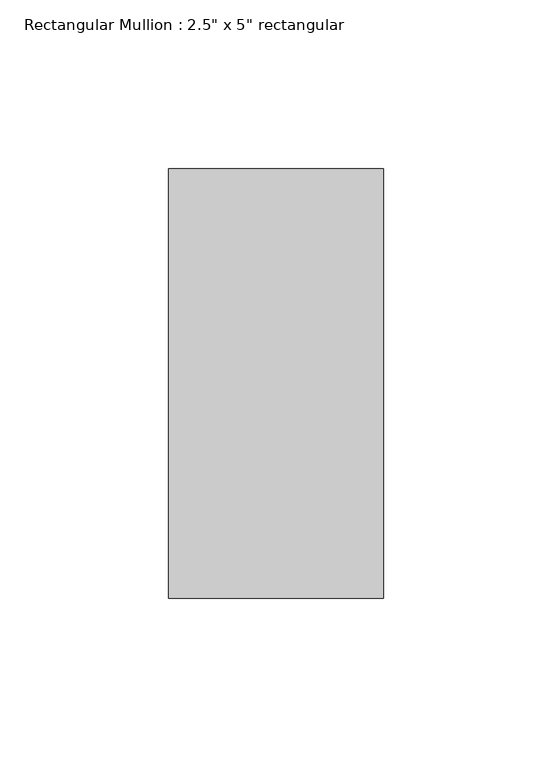
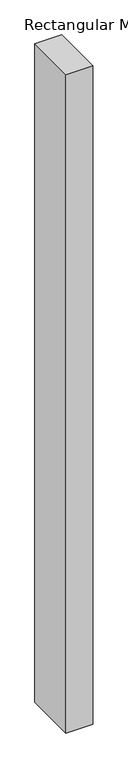
"""IFC4 building model written with IfcOpenShell, lengths in millimetres: member geometry."""

from ifc_helpers import new_model, si_unit, frame, origin, place, context, project, spatial, polyline, outline, extrude, source, transform, mapped, element, save


def member_36da3e1e(model_context):
    return source(origin(), model_context, "Body", "SweptSolid", [
        extrude(outline(polyline([(0.0, 63.5), (0.0, -63.5), (-63.5, -63.5), (-63.5, 63.5), (0.0, 63.5)])), frame((0.0, 0.0, -1645.4701172), z_axis=(0.0, 0.0, 1.0), x_axis=(1.0, 0.0, 0.0)), (0.0, 0.0, 1.0), 1645.4701172),
    ])


if __name__ == "__main__":
    model = new_model("IFC4")
    model_context = context("Model", 3, world=origin())
    ifc_project = project(units=[si_unit("LENGTHUNIT", "METRE", prefix="MILLI")], contexts=[model_context])
    site = spatial("IfcSite", under=ifc_project)
    building = spatial("IfcBuilding", under=site)
    placement = place(None, origin())
    member_shape = member_36da3e1e(model_context)
    element("IfcMember", 1, ObjectType="Rectangular Mullion : 2.5\" x 5\" rectangular", at=placement, inside=building, context=model_context, shape_type="MappedRepresentation", body=[
        mapped(member_shape, transform((0.0, 0.0, 0.0), x_axis=(1.0, 0.0, 0.0), y_axis=(0.0, 1.0, 0.0), z_axis=(0.0, 0.0, 1.0))),
    ])
    save(model, "model.ifc")

# Revit data of these elements
# Type "Rectangular Mullion : 2.5\" x 5\" rectangular"
#   built-in parameter 1007304 = 0.416667 (stored number, unit not read)
#   built-in parameter 1007301 = 0.104167 (stored number, unit not read)
#   built-in parameter 1007300 = 0.104167 (stored number, unit not read)
# Element 1 (IfcMember, "Rectangular Mullion : 2.5\" x 5\" rectangular")
#   Materials on its faces: "Aluminum"
# Materials
#   "Aluminum": class "Metal", colour RGB 247 247 247, transparency 0, Description = "Aluminum 6061", Cost = 0
